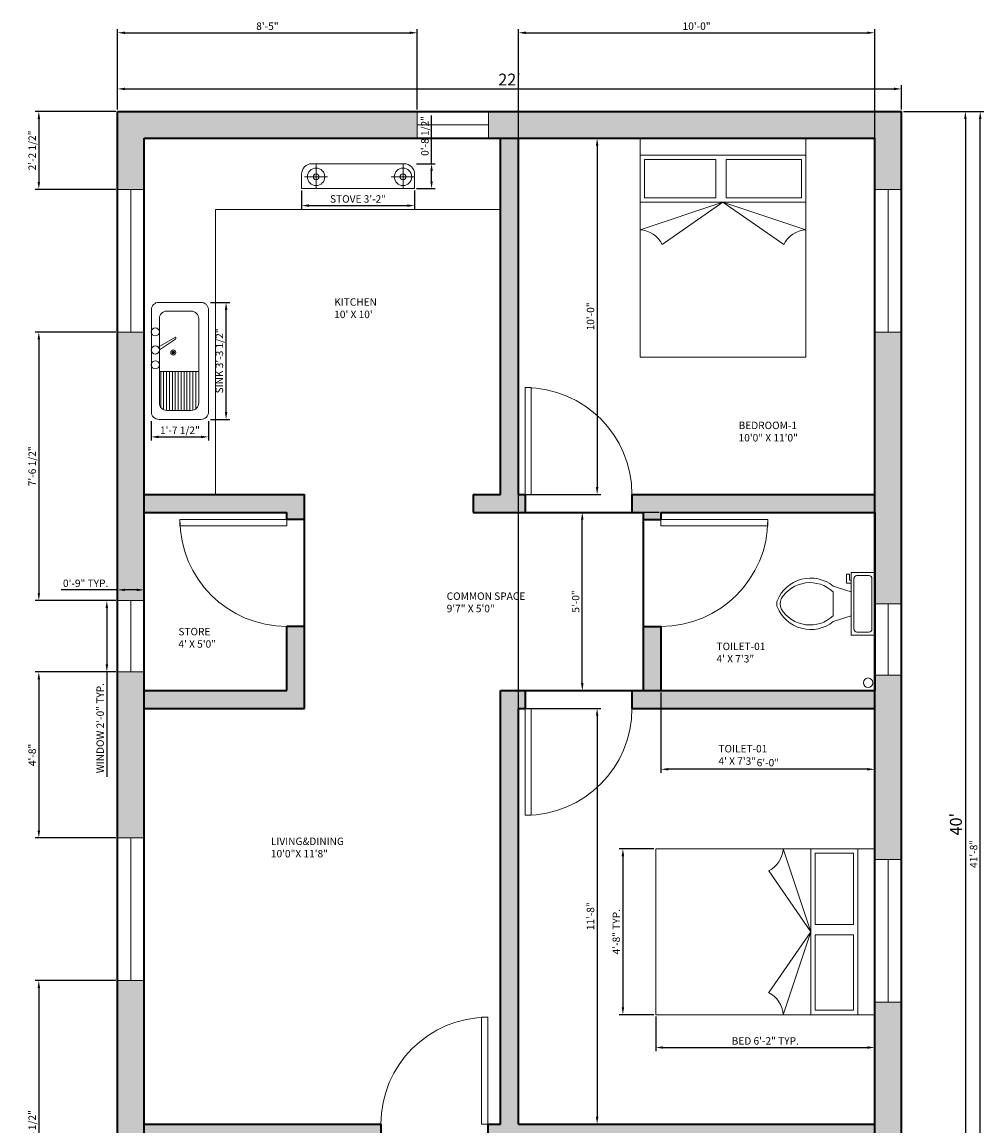
# Model space of a CAD drawing. Units: inches. Extents: x 5395 to 6469, y -203 to 448.
# Tile 7 of 7: x 6145 to 6469, y -16 to 355. Entities that reach past the tile are written whole.
import ezdxf

# ---------------------------------------------------------------- set-up
doc = ezdxf.new("R2010")
doc.units = ezdxf.units.IN
for name, color, linetype, lineweight in [('A-ANNO-DIMS', 2, 'Continuous', 18), ('A-AREA-IDEN', 6, 'Continuous', 18), ('A-EQPM', 70, 'Continuous', 18), ('A-FLOR-CASE', 32, 'Continuous', 18), ('A-FLOR-FIXT', 70, 'Continuous', 18), ('A-GLAZ', 4, 'Continuous', 18), ('A-WALL', 7, 'Continuous', 35), ('A-WALL-PATT', 11, 'Continuous', 9), ('door', 240, 'Continuous', 18), ('furniture', 70, 'Continuous', 18)]:
    doc.layers.add(name, color=color, linetype=linetype, lineweight=lineweight)
doc.styles.get("Standard").update_dxf_attribs({"font": 'arial.ttf'})
doc.dimstyles.new('ISO-25', dxfattribs={"dimtxt": 2.5, "dimasz": 2.5, "dimexe": 1.25, "dimexo": 0.625, "dimtad": 1, "dimdec": 1, "dimlunit": 3, "dimtxsty": 'Standard', "dimcen": 2.5, "dimadec": 0, "dimazin": 0, "dimtfac": 1, "dimtdec": 1, "dimtmove": 0, "dimatfit": 3, "dimfxl": 1, "dimarcsym": 0})

# ---------------------------------------------------------------- blocks, each defined once
blk = doc.blocks.new('*U2')
for p, q in [((0, 0), (0, -5)), ((30, 0), (30, -5))]:
    blk.add_line(p, q)
blk.add_lwpolyline([(0, 0), (0, 30), (1.75, 30), (1.75, 0)], close=True)
blk.add_arc((0, 0), 30, 0, 90)
blk = doc.blocks.new('*U4')
for p, q in [((0, 0), (0, 5)), ((30, 0), (30, 5))]:
    blk.add_line(p, q)
blk.add_lwpolyline([(0, 0), (0, -30), (1.75, -30), (1.75, 0)], close=True)
blk.add_arc((0, 0), 30, 270, 0)
blk = doc.blocks.new('*U3')
for p, q in [((-30, 0), (-30, -5)), ((0, 0), (0, -5))]:
    blk.add_line(p, q)
blk.add_lwpolyline([(0, 0), (0, 30), (-1.75, 30), (-1.75, 0)], close=True)
blk.add_arc((0, 0), 30, 90, 180)
blk = doc.blocks.new('*U5')
for p, q in [((-30, 0), (-30, 5)), ((0, 0), (0, 5))]:
    blk.add_line(p, q)
blk.add_lwpolyline([(0, 0), (0, -30), (-1.75, -30), (-1.75, 0)], close=True)
blk.add_arc((0, 0), 30, 180, 270)
blk = doc.blocks.new('*U26')
for p, q in [((0, 0), (0, -5)), ((-30, 0), (-30, -5))]:
    blk.add_line(p, q)
blk.add_lwpolyline([(0, 0), (0, 30), (-1.75, 30), (-1.75, 0)], close=True)
blk.add_arc((0, 0), 30, 90, 180)
blk = doc.blocks.new('sink')
for p, q in [((-11.38, 27.19), (-5.63, 30.57)), ((-11.01, 26.26), (-5.62, 29.92)), ((-11.03, 19), (2.23, 19)), ((-10.58, 19), (-10.58, 7)), ((-9.6, 19), (-9.6, 6.16)), ((-8.61, 19), (-8.61, 5.92)), ((-7.63, 19), (-7.63, 5.92)), ((-6.64, 19), (-6.64, 5.92)), ((-5.66, 19), (-5.66, 5.92)), ((-4.67, 19), (-4.67, 5.92)), ((-3.69, 19), (-3.69, 5.92)), ((-2.7, 19), (-2.7, 5.92)), ((-1.72, 19), (-1.72, 5.92)), ((-0.73, 19), (-0.73, 5.92)), ((0.25, 19), (0.25, 5.98)), ((1.23, 19), (1.23, 6.43))]:
    blk.add_line(p, q)
for points in [[(-11.21, 42.26), (3.04, 42.26, -0.414214), (5.54, 39.76), (5.54, 5.38, -0.414214), (3.04, 2.88), (-11.21, 2.88, -0.414214), (-13.71, 5.38), (-13.71, 39.76, -0.414214)], [(-8.53, 39.31), (-0.27, 39.31, -0.414214), (2.23, 36.81), (2.23, 8.42, -0.414214), (-0.27, 5.92), (-8.53, 5.92, -0.414214), (-11.03, 8.42), (-11.03, 36.81, -0.414214)]]:
    blk.add_lwpolyline(points, format="xyb", close=True)
for centre, radius in [((-12.38, 32.33), 1.37), ((-12.38, 26.26), 1.37), ((-6.32, 25.41), 0.854), ((-12.38, 21.24), 1.37), ((-6.32, 25.41), 0.432), ((-6.32, 25.41), 0.203)]:
    blk.add_circle(centre, radius)
blk.add_arc((-5.86, 30.24), 0.398, 306.1138, 55.3114)
blk = doc.blocks.new('modern bed')
for p, q in [((-55.85, 73.76), (-55.85, 0)), ((0, 0), (0, 73.76)), ((-55.85, 68.07), (0, 68.07)), ((-54.35, 66.57), (-54.35, 53.68)), ((-54.35, 66.57), (-30.33, 66.57)), ((-30.33, 66.57), (-30.33, 53.68)), ((-26.87, 66.57), (-1.5, 66.57)), ((-26.87, 66.57), (-26.87, 53.68)), ((-1.5, 53.68), (-1.5, 66.57)), ((-55.85, 52.18), (0, 52.18)), ((-27.93, 52.18), (-55.85, 42.95)), ((-54.35, 53.68), (-30.33, 53.68)), ((-27.93, 52.18), (-48.41, 38.03)), ((-27.93, 52.18), (0, 42.95)), ((-27.93, 52.18), (-7.44, 38.03)), ((-26.87, 53.68), (-1.5, 53.68)), ((-55.85, 0), (0, 0))]:
    blk.add_line(p, q)
blk.add_lwpolyline([(-55.85, 73.76), (0, 73.76)])
for centre, start, end in [((-56.5, 33.89), 27.0819, 85.9278), ((0.64, 33.89), 94.0722, 152.9181)]:
    blk.add_arc(centre, 9.08, start, end)
blk = doc.blocks.new('Toilet - top')
for p, q in [((9.5, -6), (9.5, -2)), ((-10, -8.5), (-8, -8.5)), ((-10, -9.5), (-10, -8.5)), ((-7, -9.5), (-10, -9.5)), ((-8, -8.5), (-8, -8)), ((-7, -8), (-7, -9.5)), ((-4, -8), (-6, -14)), ((4, -8), (6, -14)), ((4, -14), (-4, -14))]:
    blk.add_line(p, q)
blk.add_lwpolyline([(10.5, -8), (10.5, 0), (-10.5, 0), (-10.5, -8)], close=True)
for points in [[(-9.5, -2), (-9.5, -6)], [(8.5, -1), (-8.5, -1)], [(-8.5, -7), (8.5, -7)]]:
    blk.add_lwpolyline(points)
for centre, radius, start, end in [((-8.62, -1.88), 0.884, 81.8699, 188.1301), ((8.62, -1.88), 0.884, 351.8699, 98.1301), ((-8.62, -6.12), 0.884, 171.8699, 278.1301), ((8.62, -6.12), 0.884, 261.8699, 8.1301), ((3.52, -21.58), 12.17, 141.4691, 247.9714), ((4.2, -21.82), 11.33, 136.3677, 238.9468), ((-3.52, -21.58), 12.17, 292.0284, 38.5307), ((-4.2, -21.82), 11.33, 301.053, 43.6321), ((0, -27.88), 4, 245.7318, 294.2682), ((0, -29), 4, 254.8605, 285.1395)]:
    blk.add_arc(centre, radius, start, end)
blk = doc.blocks.new('*D27')
at = {"layer": 'A-ANNO-DIMS', "color": 0, "lineweight": -2, "transparency": 16777216}
for p, q in [((6177.33, 325.93), (6177.33, 334.16)), ((6179.83, 332.91), (6438.83, 332.91)), ((6441.33, 325.93), (6441.33, 334.16))]:
    blk.add_line(p, q, dxfattribs=at)
at = {"layer": 'A-ANNO-DIMS', "color": 0, "transparency": 16777216}
for points in [[(6179.83, 333.33), (6179.83, 332.49), (6177.33, 332.91)], [(6438.83, 333.33), (6438.83, 332.49), (6441.33, 332.91)]]:
    blk.add_solid(points, dxfattribs=at)
at = {"layer": 'Defpoints', "color": 0, "transparency": 16777216}
for p in [(6441.33, 332.91), (6177.33, 325.31), (6441.33, 325.31)]:
    blk.add_point(p, dxfattribs=at)
at = {"layer": 'A-ANNO-DIMS', "color": 0, "transparency": 16777216, "insert": (6309.33, 335.54), "char_height": 4, "attachment_point": 5}
blk.add_mtext("22'", dxfattribs=at)
blk = doc.blocks.new('STOVE')
for p, q in [((-46.84, 5.62), (-46.82, 11.55)), ((-5.51, 5.62), (-5.49, 11.55)), ((-46.84, 5.62), (-52.42, 5.62)), ((-46.84, 5.62), (-46.84, 0.29)), ((-46.84, 5.62), (-41.4, 5.62)), ((-5.51, 5.62), (-11.1, 5.62)), ((-5.51, 5.62), (-5.51, 0.29)), ((-5.51, 5.62), (-0.08, 5.62))]:
    blk.add_line(p, q)
blk.add_lwpolyline([(-48.78, 11.85), (-5, 11.85, -0.414214), (0, 6.85), (0, 0), (-53.78, 0), (-53.78, 6.85, -0.414214)], format="xyb", close=True)
for centre, radius in [((-46.84, 5.62), 4.14), ((-46.84, 5.62), 1.41), ((-5.51, 5.62), 4.14), ((-5.51, 5.62), 1.41)]:
    blk.add_circle(centre, radius)
blk = doc.blocks.new('*D28')
at = {"layer": 'A-ANNO-DIMS', "color": 0, "lineweight": -2, "transparency": 16777216}
for p, q in [((6441.96, 325.31), (6464.09, 325.31)), ((6462.84, 322.81), (6462.84, -152.19)), ((6441.96, -154.69), (6464.09, -154.69))]:
    blk.add_line(p, q, dxfattribs=at)
at = {"layer": 'A-ANNO-DIMS', "color": 0, "transparency": 16777216}
for points in [[(6462.42, 322.81), (6463.25, 322.81), (6462.84, 325.31)], [(6462.42, -152.19), (6463.25, -152.19), (6462.84, -154.69)]]:
    blk.add_solid(points, dxfattribs=at)
at = {"layer": 'Defpoints', "color": 0, "transparency": 16777216}
for p in [(6441.33, 325.31), (6441.33, -154.69), (6462.84, -154.69)]:
    blk.add_point(p, dxfattribs=at)
at = {"layer": 'A-ANNO-DIMS', "color": 0, "transparency": 16777216, "insert": (6460.17, 85.31), "char_height": 4, "attachment_point": 5, "rotation": 90}
blk.add_mtext("40'", dxfattribs=at)
blk = doc.blocks.new('WINDOW-48IN')
for p, q in [((0, 0), (0, 9)), ((48, 0), (48, 9)), ((0, 4.5), (48, 4.5))]:
    blk.add_line(p, q)
blk = doc.blocks.new('WINDOW-24IN')
for p, q in [((0, 24), (9, 24)), ((4.5, 0), (4.5, 24)), ((0, 0), (9, 0))]:
    blk.add_line(p, q)
blk = doc.blocks.new('*D33')
at = {"layer": 'A-ANNO-DIMS', "color": 0, "lineweight": -2, "transparency": 16777216}
for p, q in [((6176.71, 160.61), (6172.48, 160.61)), ((6173.73, 158.11), (6173.73, 139.11)), ((6176.71, 136.61), (6172.48, 136.61)), ((6173.73, 136.61), (6173.73, 101.23))]:
    blk.add_line(p, q, dxfattribs=at)
at = {"layer": 'A-ANNO-DIMS', "color": 0, "transparency": 16777216}
for points in [[(6173.32, 158.11), (6174.15, 158.11), (6173.73, 160.61)], [(6173.32, 139.11), (6174.15, 139.11), (6173.73, 136.61)]]:
    blk.add_solid(points, dxfattribs=at)
at = {"layer": 'Defpoints', "color": 0, "transparency": 16777216}
for p in [(6177.33, 160.61), (6173.73, 136.61), (6177.33, 136.61)]:
    blk.add_point(p, dxfattribs=at)
at = {"layer": 'A-ANNO-DIMS', "color": 0, "transparency": 16777216, "insert": (6171.82, 117.67), "char_height": 2.5, "attachment_point": 5, "rotation": 90}
blk.add_mtext('WINDOW 2\'-0" TYP.', dxfattribs=at)
blk = doc.blocks.new('*D34')
at = {"layer": 'A-ANNO-DIMS', "color": 0, "lineweight": -2, "transparency": 16777216}
for p, q in [((6177.33, 164.21), (6158.35, 164.21)), ((6177.33, 161.24), (6177.33, 165.46)), ((6183.83, 164.21), (6179.83, 164.21)), ((6186.33, 161.24), (6186.33, 165.46))]:
    blk.add_line(p, q, dxfattribs=at)
at = {"layer": 'A-ANNO-DIMS', "color": 0, "transparency": 16777216}
for points in [[(6179.83, 164.63), (6179.83, 163.8), (6177.33, 164.21)], [(6183.83, 164.63), (6183.83, 163.8), (6186.33, 164.21)]]:
    blk.add_solid(points, dxfattribs=at)
at = {"layer": 'Defpoints', "color": 0, "transparency": 16777216}
for p in [(6177.33, 164.21), (6177.33, 160.61), (6186.33, 160.61)]:
    blk.add_point(p, dxfattribs=at)
at = {"layer": 'A-ANNO-DIMS', "color": 0, "transparency": 16777216, "insert": (6166.59, 166.11), "char_height": 2.5, "attachment_point": 5}
blk.add_mtext('0\'-9" TYP.', dxfattribs=at)
blk = doc.blocks.new('*D35')
at = {"layer": 'A-ANNO-DIMS', "color": 0, "lineweight": -2, "transparency": 16777216}
for p, q in [((6358.57, 20.56), (6358.57, 8.87)), ((6432.33, 20.56), (6432.33, 8.87)), ((6361.07, 10.12), (6429.83, 10.12))]:
    blk.add_line(p, q, dxfattribs=at)
at = {"layer": 'A-ANNO-DIMS', "color": 0, "transparency": 16777216}
for points in [[(6361.07, 10.54), (6361.07, 9.7), (6358.57, 10.12)], [(6429.83, 10.54), (6429.83, 9.7), (6432.33, 10.12)]]:
    blk.add_solid(points, dxfattribs=at)
at = {"layer": 'Defpoints', "color": 0, "transparency": 16777216}
for p in [(6358.57, 21.18), (6432.33, 21.18), (6432.33, 10.12)]:
    blk.add_point(p, dxfattribs=at)
at = {"layer": 'A-ANNO-DIMS', "color": 0, "transparency": 16777216, "insert": (6395.45, 12.02), "char_height": 2.5, "attachment_point": 5}
blk.add_mtext('BED 6\'-2" TYP.', dxfattribs=at)
blk = doc.blocks.new('*D36')
at = {"layer": 'A-ANNO-DIMS', "color": 0, "lineweight": -2, "transparency": 16777216}
for p, q in [((6357.95, 77.04), (6346.26, 77.04)), ((6347.51, 74.54), (6347.51, 23.68)), ((6357.95, 21.18), (6346.26, 21.18))]:
    blk.add_line(p, q, dxfattribs=at)
at = {"layer": 'A-ANNO-DIMS', "color": 0, "transparency": 16777216}
for points in [[(6347.09, 74.54), (6347.93, 74.54), (6347.51, 77.04)], [(6347.09, 23.68), (6347.93, 23.68), (6347.51, 21.18)]]:
    blk.add_solid(points, dxfattribs=at)
at = {"layer": 'Defpoints', "color": 0, "transparency": 16777216}
for p in [(6358.57, 77.04), (6347.51, 21.18), (6358.57, 21.18)]:
    blk.add_point(p, dxfattribs=at)
at = {"layer": 'A-ANNO-DIMS', "color": 0, "transparency": 16777216, "insert": (6345.61, 49.11), "char_height": 2.5, "attachment_point": 5, "rotation": 90}
blk.add_mtext('4\'-8" TYP.', dxfattribs=at)
blk = doc.blocks.new('*D39')
at = {"layer": 'A-ANNO-DIMS', "color": 0, "lineweight": -2, "transparency": 16777216}
for p, q in [((6208.61, 261.01), (6215.14, 261.01)), ((6213.89, 224.13), (6213.89, 258.51)), ((6208.61, 221.63), (6215.14, 221.63))]:
    blk.add_line(p, q, dxfattribs=at)
at = {"layer": 'A-ANNO-DIMS', "color": 0, "transparency": 16777216}
for points in [[(6213.47, 258.51), (6214.31, 258.51), (6213.89, 261.01)], [(6213.47, 224.13), (6214.31, 224.13), (6213.89, 221.63)]]:
    blk.add_solid(points, dxfattribs=at)
at = {"layer": 'Defpoints', "color": 0, "transparency": 16777216}
for p in [(6207.98, 261.01), (6213.89, 261.01), (6207.98, 221.63)]:
    blk.add_point(p, dxfattribs=at)
at = {"layer": 'A-ANNO-DIMS', "color": 0, "transparency": 16777216, "insert": (6211.97, 241.32), "char_height": 2.5, "attachment_point": 5, "rotation": 90}
blk.add_mtext('SINK 3\'-3 1/2"', dxfattribs=at)
blk = doc.blocks.new('*D40')
at = {"layer": 'A-ANNO-DIMS', "color": 0, "lineweight": -2, "transparency": 16777216}
for p, q in [((6188.69, 221), (6188.69, 214.47)), ((6207.98, 221), (6207.98, 214.47)), ((6191.19, 215.72), (6205.48, 215.72))]:
    blk.add_line(p, q, dxfattribs=at)
at = {"layer": 'A-ANNO-DIMS', "color": 0, "transparency": 16777216}
for points in [[(6191.19, 216.14), (6191.19, 215.3), (6188.69, 215.72)], [(6205.48, 216.14), (6205.48, 215.3), (6207.98, 215.72)]]:
    blk.add_solid(points, dxfattribs=at)
at = {"layer": 'Defpoints', "color": 0, "transparency": 16777216}
for p in [(6188.69, 221.63), (6207.98, 221.63), (6207.98, 215.72)]:
    blk.add_point(p, dxfattribs=at)
at = {"layer": 'A-ANNO-DIMS', "color": 0, "transparency": 16777216, "insert": (6198.34, 217.64), "char_height": 2.5, "attachment_point": 5}
blk.add_mtext('1\'-7 1/2"', dxfattribs=at)
blk = doc.blocks.new('*D45')
at = {"layer": 'A-ANNO-DIMS', "color": 0, "lineweight": -2, "transparency": 16777216}
for p, q in [((6239.3, 298.69), (6239.3, 292.36)), ((6277.37, 298.69), (6277.37, 292.36)), ((6241.8, 293.61), (6274.87, 293.61))]:
    blk.add_line(p, q, dxfattribs=at)
at = {"layer": 'A-ANNO-DIMS', "color": 0, "transparency": 16777216}
for points in [[(6241.8, 294.03), (6241.8, 293.19), (6239.3, 293.61)], [(6274.87, 294.03), (6274.87, 293.19), (6277.37, 293.61)]]:
    blk.add_solid(points, dxfattribs=at)
at = {"layer": 'Defpoints', "color": 0, "transparency": 16777216}
for p in [(6239.3, 299.32), (6277.37, 299.32), (6277.37, 293.61)]:
    blk.add_point(p, dxfattribs=at)
at = {"layer": 'A-ANNO-DIMS', "color": 0, "transparency": 16777216, "insert": (6258.33, 295.53), "char_height": 2.5, "attachment_point": 5}
blk.add_mtext('STOVE 3\'-2"', dxfattribs=at)
blk = doc.blocks.new('*D46')
at = {"layer": 'A-ANNO-DIMS', "color": 0, "lineweight": -2, "transparency": 16777216}
for p, q in [((6283.08, 307.71), (6283.08, 323.93)), ((6277.99, 307.71), (6284.33, 307.71)), ((6283.08, 301.82), (6283.08, 305.21)), ((6277.99, 299.32), (6284.33, 299.32))]:
    blk.add_line(p, q, dxfattribs=at)
at = {"layer": 'A-ANNO-DIMS', "color": 0, "transparency": 16777216}
for points in [[(6282.66, 305.21), (6283.49, 305.21), (6283.08, 307.71)], [(6282.66, 301.82), (6283.49, 301.82), (6283.08, 299.32)]]:
    blk.add_solid(points, dxfattribs=at)
at = {"layer": 'Defpoints', "color": 0, "transparency": 16777216}
for p in [(6277.37, 307.71), (6283.08, 307.71), (6277.37, 299.32)]:
    blk.add_point(p, dxfattribs=at)
at = {"layer": 'A-ANNO-DIMS', "color": 0, "transparency": 16777216, "insert": (6281.16, 317.07), "char_height": 2.5, "attachment_point": 5, "rotation": 90}
blk.add_mtext('0\'-8 1/2"', dxfattribs=at)
blk = doc.blocks.new('*D73')
at = {"layer": 'A-ANNO-DIMS', "color": 0, "lineweight": -2, "transparency": 16777216}
for p, q in [((6177.33, 325.93), (6177.33, 353.06)), ((6179.83, 351.81), (6275.76, 351.81)), ((6278.26, 325.93), (6278.26, 353.06))]:
    blk.add_line(p, q, dxfattribs=at)
at = {"layer": 'A-ANNO-DIMS', "color": 0, "transparency": 16777216}
for points in [[(6179.83, 352.22), (6179.83, 351.39), (6177.33, 351.81)], [(6275.76, 352.22), (6275.76, 351.39), (6278.26, 351.81)]]:
    blk.add_solid(points, dxfattribs=at)
at = {"layer": 'Defpoints', "color": 0, "transparency": 16777216}
for p in [(6278.26, 351.81), (6177.33, 325.31), (6278.26, 325.31)]:
    blk.add_point(p, dxfattribs=at)
at = {"layer": 'A-ANNO-DIMS', "color": 0, "transparency": 16777216, "insert": (6227.8, 353.71), "char_height": 2.5, "attachment_point": 5}
blk.add_mtext('8\'-5"', dxfattribs=at)
blk = doc.blocks.new('*D74')
at = {"layer": 'A-ANNO-DIMS', "color": 0, "lineweight": -2, "transparency": 16777216}
for p, q in [((6176.71, 325.31), (6149.58, 325.31)), ((6150.83, 322.81), (6150.83, 301.55)), ((6176.71, 299.05), (6149.58, 299.05))]:
    blk.add_line(p, q, dxfattribs=at)
at = {"layer": 'A-ANNO-DIMS', "color": 0, "transparency": 16777216}
for points in [[(6150.42, 322.81), (6151.25, 322.81), (6150.83, 325.31)], [(6150.42, 301.55), (6151.25, 301.55), (6150.83, 299.05)]]:
    blk.add_solid(points, dxfattribs=at)
at = {"layer": 'Defpoints', "color": 0, "transparency": 16777216}
for p in [(6177.33, 325.31), (6150.83, 299.05), (6177.33, 299.05)]:
    blk.add_point(p, dxfattribs=at)
at = {"layer": 'A-ANNO-DIMS', "color": 0, "transparency": 16777216, "insert": (6148.92, 312.18), "char_height": 2.5, "attachment_point": 5, "rotation": 90}
blk.add_mtext('2\'-2 1/2"', dxfattribs=at)
blk = doc.blocks.new('*D75')
at = {"layer": 'A-ANNO-DIMS', "color": 0, "lineweight": -2, "transparency": 16777216}
for p, q in [((6176.71, 251.05), (6149.58, 251.05)), ((6150.83, 248.55), (6150.83, 163.11)), ((6176.71, 160.61), (6149.58, 160.61))]:
    blk.add_line(p, q, dxfattribs=at)
at = {"layer": 'A-ANNO-DIMS', "color": 0, "transparency": 16777216}
for points in [[(6150.42, 248.55), (6151.25, 248.55), (6150.83, 251.05)], [(6150.42, 163.11), (6151.25, 163.11), (6150.83, 160.61)]]:
    blk.add_solid(points, dxfattribs=at)
at = {"layer": 'Defpoints', "color": 0, "transparency": 16777216}
for p in [(6177.33, 251.05), (6150.83, 160.61), (6177.33, 160.61)]:
    blk.add_point(p, dxfattribs=at)
at = {"layer": 'A-ANNO-DIMS', "color": 0, "transparency": 16777216, "insert": (6148.92, 205.83), "char_height": 2.5, "attachment_point": 5, "rotation": 90}
blk.add_mtext('7\'-6 1/2"', dxfattribs=at)
blk = doc.blocks.new('*D76')
at = {"layer": 'A-ANNO-DIMS', "color": 0, "lineweight": -2, "transparency": 16777216}
for p, q in [((6176.71, 136.61), (6149.58, 136.61)), ((6150.83, 134.11), (6150.83, 83.17)), ((6176.71, 80.67), (6149.58, 80.67))]:
    blk.add_line(p, q, dxfattribs=at)
at = {"layer": 'A-ANNO-DIMS', "color": 0, "transparency": 16777216}
for points in [[(6150.42, 134.11), (6151.25, 134.11), (6150.83, 136.61)], [(6150.42, 83.17), (6151.25, 83.17), (6150.83, 80.67)]]:
    blk.add_solid(points, dxfattribs=at)
at = {"layer": 'Defpoints', "color": 0, "transparency": 16777216}
for p in [(6177.33, 136.61), (6150.83, 80.67), (6177.33, 80.67)]:
    blk.add_point(p, dxfattribs=at)
at = {"layer": 'A-ANNO-DIMS', "color": 0, "transparency": 16777216, "insert": (6148.93, 108.64), "char_height": 2.5, "attachment_point": 5, "rotation": 90}
blk.add_mtext('4\'-8"', dxfattribs=at)
blk = doc.blocks.new('*D77')
at = {"layer": 'A-ANNO-DIMS', "color": 0, "lineweight": -2, "transparency": 16777216}
for p, q in [((6176.71, 32.67), (6149.58, 32.67)), ((6150.83, 30.17), (6150.83, -65.51)), ((6176.71, -68.01), (6149.58, -68.01))]:
    blk.add_line(p, q, dxfattribs=at)
at = {"layer": 'A-ANNO-DIMS', "color": 0, "transparency": 16777216}
for points in [[(6150.42, 30.17), (6151.25, 30.17), (6150.83, 32.67)], [(6150.42, -65.51), (6151.25, -65.51), (6150.83, -68.01)]]:
    blk.add_solid(points, dxfattribs=at)
at = {"layer": 'Defpoints', "color": 0, "transparency": 16777216}
for p in [(6177.33, 32.67), (6150.83, -68.01), (6177.33, -68.01)]:
    blk.add_point(p, dxfattribs=at)
at = {"layer": 'A-ANNO-DIMS', "color": 0, "transparency": 16777216, "insert": (6148.92, -17.67), "char_height": 2.5, "attachment_point": 5, "rotation": 90}
blk.add_mtext('8\'-4 1/2"', dxfattribs=at)
blk = doc.blocks.new('*D81')
at = {"layer": 'A-ANNO-DIMS', "color": 0, "lineweight": -2, "transparency": 16777216}
for p, q in [((6312.33, -15.07), (6312.33, 353.06)), ((6314.83, 351.81), (6429.83, 351.81)), ((6432.33, -15.07), (6432.33, 353.06))]:
    blk.add_line(p, q, dxfattribs=at)
at = {"layer": 'A-ANNO-DIMS', "color": 0, "transparency": 16777216}
for points in [[(6314.83, 352.22), (6314.83, 351.39), (6312.33, 351.81)], [(6429.83, 352.22), (6429.83, 351.39), (6432.33, 351.81)]]:
    blk.add_solid(points, dxfattribs=at)
at = {"layer": 'Defpoints', "color": 0, "transparency": 16777216}
for p in [(6432.33, 351.81), (6312.33, -15.69), (6432.33, -15.69)]:
    blk.add_point(p, dxfattribs=at)
at = {"layer": 'A-ANNO-DIMS', "color": 0, "transparency": 16777216, "insert": (6372.33, 353.71), "char_height": 2.5, "attachment_point": 5}
blk.add_mtext('10\'-0"', dxfattribs=at)
blk = doc.blocks.new('*D82')
at = {"layer": 'A-ANNO-DIMS', "color": 0, "lineweight": -2, "transparency": 16777216}
for p, q in [((6312.96, 124.31), (6340.08, 124.31)), ((6338.83, 121.81), (6338.83, -13.19)), ((6312.96, -15.69), (6340.08, -15.69))]:
    blk.add_line(p, q, dxfattribs=at)
at = {"layer": 'A-ANNO-DIMS', "color": 0, "transparency": 16777216}
for points in [[(6338.42, 121.81), (6339.25, 121.81), (6338.83, 124.31)], [(6338.42, -13.19), (6339.25, -13.19), (6338.83, -15.69)]]:
    blk.add_solid(points, dxfattribs=at)
at = {"layer": 'Defpoints', "color": 0, "transparency": 16777216}
for p in [(6312.33, 124.31), (6312.33, -15.69), (6338.83, -15.69)]:
    blk.add_point(p, dxfattribs=at)
at = {"layer": 'A-ANNO-DIMS', "color": 0, "transparency": 16777216, "insert": (6336.93, 54.31), "char_height": 2.5, "attachment_point": 5, "rotation": 90}
blk.add_mtext('11\'-8"', dxfattribs=at)
blk = doc.blocks.new('*D83')
at = {"layer": 'A-ANNO-DIMS', "color": 0, "lineweight": -2, "transparency": 16777216}
for p, q in [((6312.96, 316.31), (6340.08, 316.31)), ((6338.83, 313.81), (6338.83, 198.81)), ((6312.96, 196.31), (6340.08, 196.31))]:
    blk.add_line(p, q, dxfattribs=at)
at = {"layer": 'A-ANNO-DIMS', "color": 0, "transparency": 16777216}
for points in [[(6338.42, 313.81), (6339.25, 313.81), (6338.83, 316.31)], [(6338.42, 198.81), (6339.25, 198.81), (6338.83, 196.31)]]:
    blk.add_solid(points, dxfattribs=at)
at = {"layer": 'Defpoints', "color": 0, "transparency": 16777216}
for p in [(6312.33, 316.31), (6312.33, 196.31), (6338.83, 196.31)]:
    blk.add_point(p, dxfattribs=at)
at = {"layer": 'A-ANNO-DIMS', "color": 0, "transparency": 16777216, "insert": (6336.93, 256.31), "char_height": 2.5, "attachment_point": 5, "rotation": 90}
blk.add_mtext('10\'-0"', dxfattribs=at)
blk = doc.blocks.new('*D84')
at = {"layer": 'A-ANNO-DIMS', "color": 0, "lineweight": -2, "transparency": 16777216}
for p, q in [((6360.33, 129.68), (6360.33, 102.56)), ((6432.33, 129.68), (6432.33, 102.56)), ((6429.83, 103.81), (6362.83, 103.81))]:
    blk.add_line(p, q, dxfattribs=at)
at = {"layer": 'A-ANNO-DIMS', "color": 0, "transparency": 16777216}
for points in [[(6362.83, 104.22), (6362.83, 103.39), (6360.33, 103.81)], [(6429.83, 104.22), (6429.83, 103.39), (6432.33, 103.81)]]:
    blk.add_solid(points, dxfattribs=at)
at = {"layer": 'Defpoints', "color": 0, "transparency": 16777216}
for p in [(6360.33, 130.31), (6432.33, 130.31), (6360.33, 103.81)]:
    blk.add_point(p, dxfattribs=at)
at = {"layer": 'A-ANNO-DIMS', "color": 0, "transparency": 16777216, "insert": (6396.33, 105.71), "char_height": 2.5, "attachment_point": 5}
blk.add_mtext('6\'-0"', dxfattribs=at)
blk = doc.blocks.new('*D85')
at = {"layer": 'A-ANNO-DIMS', "color": 0, "lineweight": -2, "transparency": 16777216}
for p, q in [((6359.71, 190.31), (6332.58, 190.31)), ((6333.83, 132.81), (6333.83, 187.81)), ((6359.71, 130.31), (6332.58, 130.31))]:
    blk.add_line(p, q, dxfattribs=at)
at = {"layer": 'A-ANNO-DIMS', "color": 0, "transparency": 16777216}
for points in [[(6333.42, 187.81), (6334.25, 187.81), (6333.83, 190.31)], [(6333.42, 132.81), (6334.25, 132.81), (6333.83, 130.31)]]:
    blk.add_solid(points, dxfattribs=at)
at = {"layer": 'Defpoints', "color": 0, "transparency": 16777216}
for p in [(6333.83, 190.31), (6360.33, 190.31), (6360.33, 130.31)]:
    blk.add_point(p, dxfattribs=at)
at = {"layer": 'A-ANNO-DIMS', "color": 0, "transparency": 16777216, "insert": (6331.93, 160.31), "char_height": 2.5, "attachment_point": 5, "rotation": 90}
blk.add_mtext('5\'-0"', dxfattribs=at)
blk = doc.blocks.new('*D88')
at = {"layer": 'A-ANNO-DIMS', "color": 0, "lineweight": -2, "transparency": 16777216}
for p, q in [((6441.96, 325.31), (6469.08, 325.31)), ((6467.83, -172.19), (6467.83, 322.81)), ((6322.98, -174.69), (6469.08, -174.69))]:
    blk.add_line(p, q, dxfattribs=at)
at = {"layer": 'A-ANNO-DIMS', "color": 0, "transparency": 16777216}
for points in [[(6467.42, 322.81), (6468.25, 322.81), (6467.83, 325.31)], [(6467.42, -172.19), (6468.25, -172.19), (6467.83, -174.69)]]:
    blk.add_solid(points, dxfattribs=at)
at = {"layer": 'Defpoints', "color": 0, "transparency": 16777216}
for p in [(6441.33, 325.31), (6467.83, 325.31), (6322.36, -174.69)]:
    blk.add_point(p, dxfattribs=at)
at = {"layer": 'A-ANNO-DIMS', "color": 0, "transparency": 16777216, "insert": (6465.93, 75.31), "char_height": 2.5, "attachment_point": 5, "rotation": 90}
blk.add_mtext('41\'-8"', dxfattribs=at)

msp = doc.modelspace()

# ---------------------------------------------------------------- hatches: boundary and pattern name
at = {"layer": 'A-WALL-PATT'}
h = msp.add_hatch(color=256, dxfattribs=at)
h.dxf.hatch_style = 1
h.paths.add_polyline_path([(6278.26, 325.31), (6177.33, 325.31), (6177.33, 299.05), (6186.33, 299.05), (6186.33, 316.31), (6278.26, 316.31)])
h.paths.add_polyline_path([(6186.33, 251.05), (6177.33, 251.05), (6177.33, 160.61), (6186.33, 160.61)])
h.paths.add_polyline_path([(6186.33, 136.61), (6177.33, 136.61), (6177.33, 80.67), (6186.33, 80.67)])
h.paths.add_polyline_path([(6240.33, 152.04), (6234.33, 152.04), (6234.33, 130.31), (6186.33, 130.31), (6186.33, 124.31), (6240.33, 124.31)])
h.paths.add_polyline_path([(6240.33, 196.31), (6186.33, 196.31), (6186.33, 190.31), (6234.33, 190.31), (6234.33, 188.04), (6240.33, 188.04)])
h.paths.add_polyline_path([(6186.33, 32.67), (6177.33, 32.67), (6177.33, -68.01), (6186.33, -68.01)])
h.paths.add_polyline_path([(6266.01, -15.69), (6186.33, -15.69), (6186.33, -21.69), (6266.01, -21.69)])
h.paths.add_polyline_path([(6186.33, -116.01), (6177.33, -116.01), (6177.33, -153.69), (6270.33, -153.69), (6270.33, -145.69), (6186.33, -145.69)])
h.paths.add_polyline_path([(6320.33, -105.69), (6314.33, -105.69), (6314.33, -145.69), (6306.33, -145.69), (6306.33, -153.69), (6320.33, -153.69)])
h.paths.add_polyline_path([(6441.33, -65.42), (6432.33, -65.42), (6432.33, -99.69), (6306.33, -99.69), (6306.33, -105.69), (6441.33, -105.69)])
h.paths.add_polyline_path([(6432.33, -15.69), (6312.33, -15.69), (6312.33, 124.31), (6314.57, 124.31), (6314.57, 130.31), (6306.33, 130.31), (6306.33, -15.69), (6302.01, -15.69), (6302.01, -21.69), (6432.33, -21.69)])
h.paths.add_polyline_path([(6441.33, 25.42), (6432.33, 25.42), (6432.33, -48.44), (6441.33, -48.44)])
h.paths.add_polyline_path([(6441.33, 135.52), (6432.33, 135.52), (6432.33, 130.31), (6432.33, 73.42), (6441.33, 73.42)])
h.paths.add_polyline_path([(6432.33, 130.31), (6350.57, 130.31), (6350.57, 124.31), (6432.33, 124.31)], flags=17)
h.paths.add_polyline_path([(6360.33, 151.9), (6354.33, 151.9), (6354.33, 130.31), (6360.33, 130.31)])
h.paths.add_polyline_path([(6441.33, 251.05), (6432.33, 251.05), (6432.33, 159.52), (6441.33, 159.52)])
h.paths.add_polyline_path([(6432.33, 196.31), (6350.57, 196.31), (6350.57, 190.31), (6354.33, 190.31), (6354.33, 187.9), (6360.33, 187.9), (6360.33, 190.31), (6432.33, 190.31)])
h.paths.add_polyline_path([(6312.33, 316.31), (6306.33, 316.31), (6306.33, 196.31), (6297.04, 196.31), (6297.04, 190.31), (6306.33, 190.31), (6314.57, 190.31), (6314.57, 196.31), (6312.33, 196.31)])
h.paths.add_polyline_path([(6441.33, 325.31), (6302.26, 325.31), (6302.26, 316.31), (6432.33, 316.31), (6432.33, 299.05), (6441.33, 299.05)])

# ---------------------------------------------------------------- linework, layer by layer
at = {"layer": 'A-FLOR-CASE'}
for points in [[(6186.33, 196.31), (6186.33, 316.31), (6306.33, 316.31)], [(6210.33, 196.31), (6210.33, 292.31), (6306.33, 292.31)]]:
    msp.add_lwpolyline(points, dxfattribs=at)
at = {"layer": 'A-FLOR-FIXT'}
msp.add_circle((6430.07, 132.96), 1.59, dxfattribs=at)
at = {"layer": 'A-WALL'}
for p, q in [((6177.33, -153.69), (6177.33, 325.31)), ((6177.33, 325.31), (6441.33, 325.31)), ((6441.33, -153.69), (6441.33, 325.31)), ((6186.33, 316.31), (6432.33, 316.31)), ((6186.33, -145.69), (6186.33, 316.31)), ((6306.33, 196.31), (6306.33, 316.31)), ((6312.33, 196.31), (6312.33, 316.31)), ((6432.33, -99.69), (6432.33, 316.31)), ((6186.33, 196.31), (6240.33, 196.31)), ((6240.33, 124.31), (6240.33, 196.31)), ((6297.04, 196.31), (6306.33, 196.31)), ((6297.04, 196.31), (6297.04, 190.31)), ((6312.33, 196.31), (6314.57, 196.31)), ((6314.57, 196.31), (6314.57, 190.31)), ((6350.57, 196.31), (6350.57, 190.31)), ((6350.57, 196.31), (6432.33, 196.31)), ((6186.33, 190.31), (6234.33, 190.31)), ((6234.33, 188.04), (6234.33, 190.31)), ((6297.04, 190.31), (6306.33, 190.31)), ((6306.33, 190.31), (6354.33, 190.31)), ((6360.33, 190.31), (6432.33, 190.31)), ((6234.33, 188.04), (6240.33, 188.04)), ((6354.33, 187.9), (6360.33, 187.9)), ((6234.33, 130.31), (6234.33, 152.04)), ((6234.33, 152.04), (6240.33, 152.04)), ((6354.33, 151.9), (6360.33, 151.9)), ((6186.33, 130.31), (6234.33, 130.31)), ((6306.33, -15.69), (6306.33, 130.31)), ((6306.33, 130.31), (6432.33, 130.31)), ((6314.57, 130.31), (6314.57, 124.31)), ((6350.57, 130.31), (6350.57, 124.31)), ((6186.33, 124.31), (6240.33, 124.31)), ((6312.33, -15.69), (6312.33, 124.31)), ((6312.33, 124.31), (6314.57, 124.31)), ((6350.57, 124.31), (6432.33, 124.31)), ((6186.33, -15.69), (6266.01, -15.69)), ((6266.01, -15.69), (6266.01, -21.69)), ((6302.01, -15.69), (6302.01, -21.69)), ((6302.01, -15.69), (6306.33, -15.69)), ((6312.33, -15.69), (6432.33, -15.69))]:
    msp.add_line(p, q, dxfattribs=at)
for points in [[(6354.33, 190.31), (6354.33, 130.31)], [(6360.33, 190.31), (6360.33, 187.9)], [(6432.33, 190.31), (6432.33, 130.31)], [(6360.33, 151.9), (6360.33, 130.31)]]:
    msp.add_lwpolyline(points, dxfattribs=at)

# ---------------------------------------------------------------- block references
at = {"layer": 'A-EQPM', "xscale": 0.7078901255405197, "yscale": 0.7078901255405197, "zscale": 0.7078901255405197}
msp.add_blockref('STOVE', (6277.37, 299.32), dxfattribs=at)
at = {"layer": 'A-FLOR-FIXT'}
msp.add_blockref('sink', (6202.44, 218.75), dxfattribs=at)
at = {"layer": 'A-FLOR-FIXT', "rotation": 270}
msp.add_blockref('Toilet - top', (6432.33, 159.52), dxfattribs=at)
at = {"layer": 'A-GLAZ'}
for name, p, rotation in [('WINDOW-24IN', (6278.26, 325.31), 270.0000000000024), ('WINDOW-48IN', (6177.33, 299.05), 269.999999999997), ('WINDOW-48IN', (6432.33, 299.05), 269.9999999999949), ('WINDOW-24IN', (6186.33, 160.61), 180), ('WINDOW-24IN', (6441.33, 159.52), 180), ('WINDOW-48IN', (6177.33, 80.67), 269.999999999997), ('WINDOW-48IN', (6432.33, 73.42), 269.9999999999949)]:
    msp.add_blockref(name, p, dxfattribs=dict(at, rotation=rotation))
at = {"layer": 'door', "xscale": 1.199999999999999, "yscale": 1.199999999999999, "zscale": 1.199999999999999}
for name, p in [('*U2', (6314.57, 196.31)), ('*U4', (6314.57, 124.31)), ('*U3', (6302.01, -15.69))]:
    msp.add_blockref(name, p, dxfattribs=at)
at = {"layer": 'door', "xscale": 1.199999999999999, "yscale": 1.199999999999999, "zscale": 1.199999999999999, "rotation": 90}
for name, p in [('*U26', (6234.33, 187.9)), ('*U5', (6360.33, 187.9))]:
    msp.add_blockref(name, p, dxfattribs=at)
at = {"layer": 'furniture'}
msp.add_blockref('modern bed', (6409.14, 242.54), dxfattribs=at)
at = {"layer": 'furniture', "rotation": 270}
msp.add_blockref('modern bed', (6358.57, 21.18), dxfattribs=at)

# ---------------------------------------------------------------- texts
at = {"layer": 'A-AREA-IDEN', "char_height": 2.5, "attachment_point": 1}
for s, insert in [("KITCHEN\\P10' X 10'", (6250.3, 262.4)), ('BEDROOM-1\\P10\'0" X 11\'0"', (6386.47, 220.85)), ('COMMON SPACE\\P9\'7" X 5\'0"', (6288.17, 163.36)), ('STORE\\P4\' X 5\'0"', (6197.83, 151.41)), ('TOILET-01\\P4\' X 7\'3"', (6379.03, 146.44)), ('TOILET-01\\P4\' X 7\'3"', (6379.69, 111.99)), ('LIVING&DINING\\P10\'0"X 11\'8"', (6228.98, 80.81))]:
    msp.add_mtext_dynamic_manual_height_columns(s, width=62.1492, gutter_width=12.5, heights=[0], dxfattribs=dict(at, insert=insert))

# ---------------------------------------------------------------- dimensions: what is measured, and where the dimension line sits
at = {"layer": 'A-ANNO-DIMS'}
for base, p1, p2, override, picture, middle in [((6278.26, 351.81), (6177.33, 325.31), (6278.26, 325.31), {"dimdec": 1, "dimlfac": 1, "dimrnd": 0, "dimzin": 1, "dimdsep": 46, "dimlunit": 4, "dimfrac": 2}, '*D73', (6227.8, 353.71)), ((6432.33, 351.81), (6312.33, -15.69), (6432.33, -15.69), {"dimdec": 1, "dimlfac": 1, "dimrnd": 0, "dimzin": 1, "dimdsep": 46, "dimlunit": 4, "dimfrac": 2}, '*D81', (6372.33, 353.71)), ((6441.33, 332.91), (6177.33, 325.31), (6441.33, 325.31), {"dimtxt": 4, "dimclrd": 0, "dimclre": 0, "dimclrt": 0}, '*D27', (6309.33, 335.54)), ((6207.98, 215.72), (6188.69, 221.63), (6207.98, 221.63), {"dimdec": 1, "dimlfac": 1, "dimrnd": 0, "dimzin": 1, "dimdsep": 46, "dimlunit": 4, "dimfrac": 2}, '*D40', (6198.34, 217.64))]:
    dim = msp.add_linear_dim(base=base, p1=p1, p2=p2, dimstyle='ISO-25', override=override, dxfattribs=at)
    dim.commit()
    dim.dimension.update_dxf_attribs({"geometry": picture, "text_midpoint": middle})
for base, p1, p2, angle, override, picture, middle in [((6150.83, 299.05), (6177.33, 325.31), (6177.33, 299.05), 90, {"dimdec": 1, "dimlfac": 1, "dimrnd": 0, "dimzin": 1, "dimdsep": 46, "dimlunit": 4, "dimfrac": 2}, '*D74', (6148.92, 312.18)), ((6283.08, 307.71), (6277.37, 299.32), (6277.37, 307.71), 90, {"dimdec": 1, "dimlfac": 1, "dimrnd": 0, "dimzin": 1, "dimdsep": 46, "dimlunit": 4, "dimfrac": 2}, '*D46', (6281.16, 317.07)), ((6467.83, 325.31), (6322.36, -174.69), (6441.33, 325.31), 90, {"dimdec": 1, "dimlfac": 1, "dimrnd": 0, "dimzin": 1, "dimdsep": 46, "dimlunit": 4, "dimfrac": 2}, '*D88', (6465.93, 75.31)), ((6462.84, -154.69), (6441.33, 325.31), (6441.33, -154.69), 90, {"dimtxt": 4, "dimclrd": 0, "dimclre": 0, "dimclrt": 0}, '*D28', (6460.17, 85.31)), ((6338.83, 196.31), (6312.33, 316.31), (6312.33, 196.31), 270, {"dimdec": 1, "dimlfac": 1, "dimrnd": 0, "dimzin": 1, "dimdsep": 46, "dimlunit": 4, "dimfrac": 2}, '*D83', (6336.93, 256.31)), ((6150.83, 160.61), (6177.33, 251.05), (6177.33, 160.61), 90, {"dimdec": 1, "dimlfac": 1, "dimrnd": 0, "dimzin": 1, "dimdsep": 46, "dimlunit": 4, "dimfrac": 2}, '*D75', (6148.92, 205.83)), ((6333.83, 190.31), (6360.33, 130.31), (6360.33, 190.31), 90, {"dimdec": 1, "dimlfac": 1, "dimrnd": 0, "dimzin": 1, "dimdsep": 46, "dimlunit": 4, "dimfrac": 2}, '*D85', (6331.93, 160.31)), ((6150.83, 80.67), (6177.33, 136.61), (6177.33, 80.67), 90, {"dimdec": 1, "dimlfac": 1, "dimrnd": 0, "dimzin": 1, "dimdsep": 46, "dimlunit": 4, "dimfrac": 2}, '*D76', (6148.93, 108.64)), ((6360.33, 103.81), (6432.33, 130.31), (6360.33, 130.31), 180, {"dimdec": 1, "dimlfac": 1, "dimrnd": 0, "dimzin": 1, "dimdsep": 46, "dimlunit": 4, "dimfrac": 2}, '*D84', (6396.33, 105.71)), ((6338.83, -15.69), (6312.33, 124.31), (6312.33, -15.69), 270, {"dimdec": 1, "dimlfac": 1, "dimrnd": 0, "dimzin": 1, "dimdsep": 46, "dimlunit": 4, "dimfrac": 2}, '*D82', (6336.93, 54.31)), ((6150.83, -68.01), (6177.33, 32.67), (6177.33, -68.01), 90, {"dimdec": 1, "dimlfac": 1, "dimrnd": 0, "dimzin": 1, "dimdsep": 46, "dimlunit": 4, "dimfrac": 2}, '*D77', (6148.92, -17.67))]:
    dim = msp.add_linear_dim(base=base, p1=p1, p2=p2, angle=angle, dimstyle='ISO-25', override=override, dxfattribs=at)
    dim.commit()
    dim.dimension.update_dxf_attribs({"geometry": picture, "text_midpoint": middle})
for base, p1, p2, text, picture, middle in [((6277.37, 293.61), (6239.3, 299.32), (6277.37, 299.32), 'STOVE <>', '*D45', (6258.33, 295.53)), ((6432.33, 10.12), (6358.57, 21.18), (6432.33, 21.18), 'BED <> TYP.', '*D35', (6395.45, 12.02))]:
    dim = msp.add_linear_dim(base=base, p1=p1, p2=p2, text=text, dimstyle='ISO-25', override={"dimdec": 1, "dimlfac": 1, "dimrnd": 0, "dimzin": 1, "dimdsep": 46, "dimlunit": 4, "dimfrac": 2}, dxfattribs=at)
    dim.commit()
    dim.dimension.update_dxf_attribs({"geometry": picture, "text_midpoint": middle})
for base, p1, p2, angle, text, picture, middle in [((6213.89, 261.01), (6207.98, 221.63), (6207.98, 261.01), 90, 'SINK <>', '*D39', (6211.97, 241.32)), ((6177.33, 164.21), (6186.33, 160.61), (6177.33, 160.61), 180, '<> TYP.', '*D34', (6166.59, 166.11)), ((6173.73, 136.61), (6177.33, 160.61), (6177.33, 136.61), 270, 'WINDOW <> TYP.', '*D33', (6171.82, 117.67)), ((6347.51, 21.18), (6358.57, 77.04), (6358.57, 21.18), 270, '<> TYP.', '*D36', (6345.61, 49.11))]:
    dim = msp.add_linear_dim(base=base, p1=p1, p2=p2, angle=angle, text=text, dimstyle='ISO-25', override={"dimdec": 1, "dimlfac": 1, "dimrnd": 0, "dimzin": 1, "dimdsep": 46, "dimlunit": 4, "dimfrac": 2}, dxfattribs=at)
    dim.commit()
    dim.dimension.update_dxf_attribs({"geometry": picture, "text_midpoint": middle})

doc.saveas('drawing.dxf')
